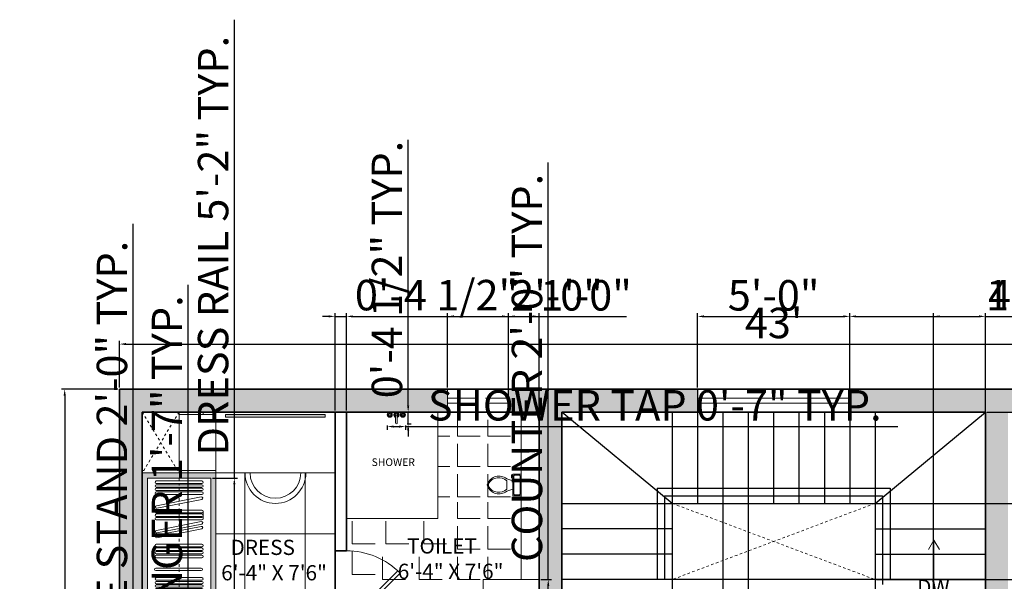
# Model space of a CAD drawing. Units: millimetres. Extents: x 542930 to 543750, y 628093 to 628738.
# Tile 7 of 14: x 542944 to 543333, y 628514 to 628735. Entities that reach past the tile are written whole.
import ezdxf

# ---------------------------------------------------------------- set-up
doc = ezdxf.new("R2010")
doc.units = ezdxf.units.MM
doc.linetypes.add('ACAD_ISO02W100', pattern=[15, 12, -3])
doc.linetypes.add('JIS_02_1.0', pattern=[2, 1, -1])
for name, color, linetype, lineweight in [('A-ANNO-DIMS', 2, 'Continuous', 18), ('A-ANNO-SYMB', 4, 'Continuous', 18), ('A-FLOR-FIXT', 9, 'Continuous', 18), ('A-FLOR-STRS', 7, 'Continuous', 25), ('A-FLOR-STRS-HIDN', 7, 'JIS_02_1.0', 13), ('A-FURN', 8, 'Continuous', 18), ('A-FURN-MILL', 8, 'Continuous', 18), ('A-FURN-MILL-HIDN', 8, 'JIS_02_1.0', 13), ('A-FURN-PATT', 9, 'Continuous', 13), ('A-GLAZ-HIDN', 70, 'ACAD_ISO02W100', 18), ('A-WALL', 7, 'Continuous', 35), ('DOORS', 30, 'Continuous', 18), ('WINDOW', 70, 'Continuous', 18)]:
    doc.layers.add(name, color=color, linetype=linetype, lineweight=lineweight)
for name, color, linetype, lineweight, true_color in [('A-ANNO-TEXT', 40, 'Continuous', 18, 0xf8d731), ('A-AREA-IDEN', 40, 'Continuous', 18, 0xf8d731), ('A-FLOR-PATT', 241, 'Continuous', 13, 0xf7abae), ('A-WALL-PATT', 251, 'Continuous', 13, 0x636466)]:
    doc.layers.add(name, color=color, linetype=linetype, lineweight=lineweight, true_color=true_color)
doc.styles.get("Standard").update_dxf_attribs({"font": 'arial.ttf'})
doc.dimstyles.new('ISO-25', dxfattribs={"dimtxt": 12, "dimasz": 2.5, "dimexe": 1.25, "dimexo": 0.625, "dimtad": 1, "dimdec": 0, "dimlunit": 3, "dimtxsty": 'Standard', "dimcen": 2.5, "dimadec": 0, "dimazin": 0, "dimtfac": 1, "dimtdec": 0, "dimtmove": 0, "dimatfit": 3, "dimfxl": 1, "dimarcsym": 0})

# ---------------------------------------------------------------- blocks, each defined once
blk = doc.blocks.new('*U3')
for p, q in [((-40, 0), (-40, -6)), ((0, 0), (0, -6))]:
    blk.add_line(p, q)
blk.add_lwpolyline([(0, 0), (-28.28, 28.28), (-29.52, 27.05), (-1.24, -1.24)], close=True)
blk.add_arc((0, 0), 40, 135, 180)
blk = doc.blocks.new('*U6')
for p, q in [((-10, -8.5), (-8, -8.5)), ((-10, -9.5), (-10, -8.5)), ((-7, -9.5), (-10, -9.5)), ((-8, -8.5), (-8, -8)), ((-7, -8), (-7, -9.5)), ((-4, -8), (-6, -14)), ((4, -8), (6, -14)), ((9.5, -6), (9.5, -2)), ((4, -14), (-4, -14))]:
    blk.add_line(p, q)
blk.add_lwpolyline([(10.5, -8), (10.5, 0), (-10.5, 0), (-10.5, -8)], close=True)
for points in [[(-9.5, -2), (-9.5, -6)], [(8.5, -1), (-8.5, -1)], [(-8.5, -7), (8.5, -7)]]:
    blk.add_lwpolyline(points)
for centre, radius, start, end in [((-8.62, -1.88), 0.884, 81.8699, 188.1301), ((-8.62, -6.12), 0.884, 171.8699, 278.1301), ((8.62, -1.88), 0.884, 351.8699, 98.1301), ((8.62, -6.12), 0.884, 261.8699, 8.1301), ((3.52, -21.58), 12.17, 141.46911, 247.97143), ((4.2, -21.82), 11.33, 136.36773, 238.94682), ((-3.52, -21.58), 12.17, 292.02843, 38.53071), ((-4.2, -21.82), 11.33, 301.05301, 43.63209), ((0, -27.88), 4, 245.73182, 294.26817), ((0, -29), 4, 254.86053, 285.13947)]:
    blk.add_arc(centre, radius, start, end)
blk = doc.blocks.new('Faucet - Bathroom top')
for p, q in [((-4.107, 0.125), (-4.375, 0.125)), ((-3.75, 0.4788), (-3.75, 0.75)), ((-3.5, 0.482), (-3.5, 0.75)), ((-3.1461, 0.125), (-2.875, 0.125)), ((3.143, 0.125), (2.875, 0.125)), ((3.5, 0.4788), (3.5, 0.75)), ((3.75, 0.482), (3.75, 0.75)), ((4.1039, 0.125), (4.375, 0.125)), ((-4.1039, -0.125), (-4.375, -0.125)), ((-3.75, -0.4821), (-3.75, -0.75)), ((-3.5, -0.4789), (-3.5, -0.75)), ((-3.143, -0.125), (-2.875, -0.125)), ((-0.5, -0.8639), (-0.5, -4.5)), ((0.5, -4.5), (0.5, -0.8631)), ((3.1461, -0.125), (2.875, -0.125)), ((3.5, -0.4821), (3.5, -0.75)), ((3.75, -0.4789), (3.75, -0.75)), ((4.107, -0.125), (4.375, -0.125))]:
    blk.add_line(p, q)
for centre, radius in [((-3.625, 0), 1.375), ((-4.625, 0), 0.2795), ((-3.625, 0), 0.5), ((-3.625, 1), 0.2795), ((-2.625, 0), 0.2795), ((0, 0), 0.5), ((3.625, 0), 1.375), ((2.625, 0), 0.2795), ((3.625, 0), 0.5), ((3.625, 1), 0.2795), ((4.625, 0), 0.2795), ((-3.625, -1), 0.2795), ((3.625, -1), 0.2795)]:
    blk.add_circle(centre, radius)
for centre, radius, start, end in [((-3.625, 0), 1, 105.2407, 164.2093), ((-3.625, 0), 1, 16.44125, 74.07887), ((0, 0), 1.5, 289.6514, 250.3603), ((0, 0), 1, 300.3431, 239.7554), ((3.625, 0), 1, 106.12, 164.0884), ((3.625, 0), 1, 16.23422, 73.90469), ((-3.625, 0), 1, 196.2342, 253.9047), ((-3.625, 0), 1, 286.12, 344.0884), ((0, -4.5), 0.5, 180, 0), ((3.625, 0), 1, 196.4413, 254.0789), ((3.625, 0), 1, 285.2407, 344.2093)]:
    blk.add_arc(centre, radius, start, end)
blk = doc.blocks.new('*D19')
at = {"layer": 'A-ANNO-DIMS', "color": 0, "lineweight": -2, "transparency": 16777216}
for p, q in [((542983.67, 628590.45), (542983.67, 628608.87)), ((542986.17, 628607.62), (543497.17, 628607.62)), ((543499.67, 628590.45), (543499.67, 628608.87))]:
    blk.add_line(p, q, dxfattribs=at)
at = {"layer": 'A-ANNO-DIMS', "color": 0, "transparency": 16777216}
for points in [[(542986.17, 628608.04), (542986.17, 628607.2), (542983.67, 628607.62)], [(543497.17, 628608.04), (543497.17, 628607.2), (543499.67, 628607.62)]]:
    blk.add_solid(points, dxfattribs=at)
at = {"layer": 'Defpoints', "color": 0, "transparency": 16777216}
for p in [(543499.67, 628607.62), (542983.67, 628589.83), (543499.67, 628589.83)]:
    blk.add_point(p, dxfattribs=at)
at = {"layer": 'A-ANNO-DIMS', "color": 0, "transparency": 16777216, "insert": (543241.67, 628614.38), "char_height": 12, "attachment_point": 5}
blk.add_mtext("43'", dxfattribs=at)
blk = doc.blocks.new('*D20')
at = {"layer": 'A-ANNO-DIMS', "color": 0, "lineweight": -2, "transparency": 16777216}
for p, q in [((542983.04, 628589.83), (542960.8, 628589.83)), ((542962.05, 628587.33), (542962.05, 628256.33)), ((542983.04, 628253.83), (542960.8, 628253.83))]:
    blk.add_line(p, q, dxfattribs=at)
at = {"layer": 'A-ANNO-DIMS', "color": 0, "transparency": 16777216}
for points in [[(542961.64, 628587.33), (542962.47, 628587.33), (542962.05, 628589.83)], [(542961.64, 628256.33), (542962.47, 628256.33), (542962.05, 628253.83)]]:
    blk.add_solid(points, dxfattribs=at)
at = {"layer": 'Defpoints', "color": 0, "transparency": 16777216}
for p in [(542983.67, 628589.83), (542962.05, 628253.83), (542983.67, 628253.83)]:
    blk.add_point(p, dxfattribs=at)
at = {"layer": 'A-ANNO-DIMS', "color": 0, "transparency": 16777216, "insert": (542955.3, 628421.83), "char_height": 12, "attachment_point": 5, "rotation": 90}
blk.add_mtext("28'", dxfattribs=at)
blk = doc.blocks.new('WARDROBE-DRESS-RAIL')
for p, q in [((0, 0), (0, 62)), ((0, 62), (25, 62)), ((3.52, 60.83), (21.52, 60.83)), ((3.52, 59.83), (21.52, 59.83)), ((3.52, 59.35), (21.52, 59.35)), ((3.52, 58.35), (21.52, 58.35)), ((25, 0), (25, 62)), ((3.52, 58.02), (21.52, 58.02)), ((3.52, 57.02), (21.52, 57.02)), ((3.52, 56.51), (21.52, 56.51)), ((3.52, 55.51), (21.52, 55.51)), ((3.57, 51.08), (21.23, 54.55)), ((3.76, 50.1), (21.43, 53.57)), ((3.52, 49.31), (21.52, 49.31)), ((3.52, 48.31), (21.52, 48.31)), ((3.52, 47.82), (21.52, 47.82)), ((3.52, 46.82), (21.52, 46.82)), ((3.52, 46.49), (21.52, 46.49)), ((3.52, 45.49), (21.52, 45.49)), ((3.57, 41.35), (21.23, 44.82)), ((3.57, 39.47), (21.23, 42.94)), ((3.76, 40.37), (21.43, 43.84)), ((3.76, 38.49), (21.43, 41.96)), ((3.52, 35.91), (21.52, 35.91)), ((3.52, 34.91), (21.52, 34.91)), ((3.52, 34.43), (21.52, 34.43)), ((3.52, 33.43), (21.52, 33.43)), ((3.52, 33.1), (21.52, 33.1)), ((3.52, 32.1), (21.52, 32.1)), ((3.52, 31.59), (21.52, 31.59)), ((3.52, 30.59), (21.52, 30.59)), ((3.27, 26.51), (21.27, 26.51)), ((3.27, 25.51), (21.27, 25.51)), ((3.52, 22.74), (21.52, 22.74)), ((3.52, 21.74), (21.52, 21.74)), ((3.52, 21.26), (21.52, 21.26)), ((3.52, 20.26), (21.52, 20.26)), ((3.52, 19.93), (21.52, 19.93)), ((3.52, 18.93), (21.52, 18.93)), ((3.52, 18.42), (21.52, 18.42)), ((3.52, 17.42), (21.52, 17.42)), ((3.56, 15.93), (21.44, 13.91)), ((3.27, 11.99), (21.27, 11.99)), ((3.44, 14.93), (21.33, 12.92)), ((3.27, 10.99), (21.27, 10.99)), ((3.52, 8.06), (21.52, 8.06)), ((3.52, 7.06), (21.52, 7.06)), ((3.52, 6.58), (21.52, 6.58)), ((3.52, 5.58), (21.52, 5.58)), ((3.52, 5.25), (21.52, 5.25)), ((3.52, 4.25), (21.52, 4.25)), ((3.52, 3.74), (21.52, 3.74)), ((3.52, 2.74), (21.52, 2.74)), ((0, 0), (25, 0))]:
    blk.add_line(p, q)
for centre, start, end in [((3.52, 60.33), 90, 270), ((3.52, 58.85), 90, 270), ((21.52, 60.33), 270, 90), ((21.52, 58.85), 270, 90), ((3.52, 57.52), 90, 270), ((3.52, 56.01), 90, 270), ((21.33, 54.06), 281.1082, 101.1082), ((21.52, 57.52), 270, 90), ((21.52, 56.01), 270, 90), ((3.67, 50.59), 101.1082, 281.1082), ((3.52, 48.81), 90, 270), ((3.52, 47.32), 90, 270), ((21.52, 48.81), 270, 90), ((21.52, 47.32), 270, 90), ((3.52, 45.99), 90, 270), ((21.33, 44.33), 281.1082, 101.1082), ((21.33, 42.45), 281.1082, 101.1082), ((21.52, 45.99), 270, 90), ((3.67, 40.86), 101.1082, 281.1082), ((3.67, 38.98), 101.1082, 281.1082), ((3.52, 35.41), 90, 270), ((21.52, 35.41), 270, 90), ((3.52, 33.93), 90, 270), ((3.52, 32.6), 90, 270), ((3.52, 31.09), 90, 270), ((21.52, 33.93), 270, 90), ((21.52, 32.6), 270, 90), ((21.52, 31.09), 270, 90), ((3.27, 26.01), 90, 270), ((21.27, 26.01), 270, 90), ((3.52, 22.24), 90, 270), ((3.52, 20.76), 90, 270), ((3.52, 19.43), 90, 270), ((21.52, 22.24), 270, 90), ((21.52, 20.76), 270, 90), ((21.52, 19.43), 270, 90), ((3.5, 15.43), 83.5593, 263.5593), ((3.52, 17.92), 90, 270), ((21.52, 17.92), 270, 90), ((3.27, 11.49), 90, 270), ((21.27, 11.49), 270, 90), ((21.39, 13.41), 263.5593, 83.5611), ((3.52, 7.56), 90, 270), ((21.52, 7.56), 270, 90), ((3.52, 6.08), 90, 270), ((3.52, 4.75), 90, 270), ((21.52, 6.08), 270, 90), ((21.52, 4.75), 270, 90), ((3.52, 3.24), 90, 270), ((21.52, 3.24), 270, 90)]:
    blk.add_arc(centre, 0.5, start, end)
blk = doc.blocks.new('SHOWER-ENCLOSURE')
for p, q in [((36, 0), (36, 42)), ((0, 0), (36, 0))]:
    blk.add_line(p, q)
blk = doc.blocks.new('LAVATORY-COUNTER')
for p, q in [((0, 0), (0, 24)), ((0, 24), (22, 24))]:
    blk.add_line(p, q)
blk = doc.blocks.new('DRESSING-STOOL')
for radius in [12, 10]:
    blk.add_arc((12, 12), radius, 180, 0)
blk = doc.blocks.new('*D31')
at = {"layer": 'A-ANNO-DIMS', "color": 0, "lineweight": -2, "transparency": 16777216}
for p, q in [((543010.77, 628478.3), (543010.77, 628630.92)), ((543012.99, 628478.3), (543009.52, 628478.3)), ((543010.77, 628461.8), (543010.77, 628475.8)), ((543012.99, 628459.3), (543009.52, 628459.3))]:
    blk.add_line(p, q, dxfattribs=at)
at = {"layer": 'A-ANNO-DIMS', "color": 0, "transparency": 16777216}
for points in [[(543010.35, 628475.8), (543011.18, 628475.8), (543010.77, 628478.3)], [(543010.35, 628461.8), (543011.18, 628461.8), (543010.77, 628459.3)]]:
    blk.add_solid(points, dxfattribs=at)
at = {"layer": 'Defpoints', "color": 0, "transparency": 16777216}
for p in [(543010.77, 628478.3), (543013.62, 628478.3), (543013.62, 628459.3)]:
    blk.add_point(p, dxfattribs=at)
at = {"layer": 'A-ANNO-DIMS', "color": 0, "transparency": 16777216, "insert": (543003.94, 628555.86), "char_height": 12, "attachment_point": 5, "rotation": 90}
blk.add_mtext('HANGER 1\'-7" TYP.', dxfattribs=at)
blk = doc.blocks.new('*D39')
at = {"layer": 'A-ANNO-DIMS', "color": 0, "lineweight": -2, "transparency": 16777216}
for p, q in [((543089.3, 628575.56), (543089.3, 628573.86)), ((543091.8, 628575.11), (543093.95, 628575.11)), ((543096.45, 628575.56), (543096.45, 628573.86)), ((543096.45, 628575.11), (543290.64, 628575.11))]:
    blk.add_line(p, q, dxfattribs=at)
at = {"layer": 'A-ANNO-DIMS', "color": 0, "transparency": 16777216}
for points in [[(543091.8, 628575.52), (543091.8, 628574.69), (543089.3, 628575.11)], [(543093.95, 628575.52), (543093.95, 628574.69), (543096.45, 628575.11)]]:
    blk.add_solid(points, dxfattribs=at)
at = {"layer": 'Defpoints', "color": 0, "transparency": 16777216}
for p in [(543089.3, 628576.18), (543096.45, 628576.18), (543096.45, 628575.11)]:
    blk.add_point(p, dxfattribs=at)
at = {"layer": 'A-ANNO-DIMS', "color": 0, "transparency": 16777216, "insert": (543194.79, 628581.94), "char_height": 12, "attachment_point": 5}
blk.add_mtext('SHOWER TAP 0\'-7" TYP.', dxfattribs=at)
blk = doc.blocks.new('*D40')
at = {"layer": 'A-ANNO-DIMS', "color": 0, "lineweight": -2, "transparency": 16777216}
for p, q in [((543097.52, 628583.33), (543097.52, 628688.18)), ((543097.07, 628580.83), (543098.77, 628580.83)), ((543097.52, 628576.18), (543097.52, 628580.83)), ((543097.07, 628576.18), (543098.77, 628576.18)), ((543097.52, 628573.68), (543097.52, 628571.18))]:
    blk.add_line(p, q, dxfattribs=at)
at = {"layer": 'A-ANNO-DIMS', "color": 0, "transparency": 16777216}
for points in [[(543097.1, 628583.33), (543097.94, 628583.33), (543097.52, 628580.83)], [(543097.1, 628573.68), (543097.94, 628573.68), (543097.52, 628576.18)]]:
    blk.add_solid(points, dxfattribs=at)
at = {"layer": 'Defpoints', "color": 0, "transparency": 16777216}
for p in [(543096.45, 628580.83), (543097.52, 628580.83), (543096.45, 628576.18)]:
    blk.add_point(p, dxfattribs=at)
at = {"layer": 'A-ANNO-DIMS', "color": 0, "transparency": 16777216, "insert": (543090.69, 628637), "char_height": 12, "attachment_point": 5, "rotation": 90}
blk.add_mtext('0\'-4 1/2" TYP.', dxfattribs=at)
blk = doc.blocks.new('*D43')
at = {"layer": 'A-ANNO-DIMS', "color": 0, "lineweight": -2, "transparency": 16777216}
for p, q in [((543028.97, 628554.83), (543028.97, 628735.47)), ((543020.29, 628554.83), (543030.22, 628554.83)), ((543028.97, 628495.33), (543028.97, 628552.33)), ((543020.29, 628492.83), (543030.22, 628492.83))]:
    blk.add_line(p, q, dxfattribs=at)
at = {"layer": 'A-ANNO-DIMS', "color": 0, "transparency": 16777216}
for points in [[(543028.55, 628552.33), (543029.38, 628552.33), (543028.97, 628554.83)], [(543028.55, 628495.33), (543029.38, 628495.33), (543028.97, 628492.83)]]:
    blk.add_solid(points, dxfattribs=at)
at = {"layer": 'Defpoints', "color": 0, "transparency": 16777216}
for p in [(543019.67, 628554.83), (543028.97, 628554.83), (543019.67, 628492.83)]:
    blk.add_point(p, dxfattribs=at)
at = {"layer": 'A-ANNO-DIMS', "color": 0, "transparency": 16777216, "insert": (543022.14, 628646.4), "char_height": 12, "attachment_point": 5, "rotation": 90}
blk.add_mtext('DRESS RAIL 5\'-2" TYP.', dxfattribs=at)
blk = doc.blocks.new('*D55')
at = {"layer": 'A-ANNO-DIMS', "color": 0, "lineweight": -2, "transparency": 16777216}
for p, q in [((543152.77, 628514.83), (543152.77, 628679.13)), ((543149.79, 628514.83), (543154.02, 628514.83)), ((543152.77, 628493.33), (543152.77, 628512.33)), ((543149.79, 628490.83), (543154.02, 628490.83))]:
    blk.add_line(p, q, dxfattribs=at)
at = {"layer": 'A-ANNO-DIMS', "color": 0, "transparency": 16777216}
for points in [[(543152.35, 628512.33), (543153.18, 628512.33), (543152.77, 628514.83)], [(543152.35, 628493.33), (543153.18, 628493.33), (543152.77, 628490.83)]]:
    blk.add_solid(points, dxfattribs=at)
at = {"layer": 'Defpoints', "color": 0, "transparency": 16777216}
for p in [(543149.17, 628514.83), (543152.77, 628514.83), (543149.17, 628490.83)]:
    blk.add_point(p, dxfattribs=at)
at = {"layer": 'A-ANNO-DIMS', "color": 0, "transparency": 16777216, "insert": (543145.93, 628598.23), "char_height": 12, "attachment_point": 5, "rotation": 90}
blk.add_mtext('COUNTER 2\'-0" TYP.', dxfattribs=at)
blk = doc.blocks.new('*D59')
at = {"layer": 'A-ANNO-DIMS', "color": 0, "lineweight": -2, "transparency": 16777216}
for p, q in [((542989.07, 628438.89), (542989.07, 628654.99)), ((542992.04, 628438.89), (542987.82, 628438.89)), ((542989.07, 628417.39), (542989.07, 628436.39)), ((542992.04, 628414.89), (542987.82, 628414.89))]:
    blk.add_line(p, q, dxfattribs=at)
at = {"layer": 'A-ANNO-DIMS', "color": 0, "transparency": 16777216}
for points in [[(542988.65, 628436.39), (542989.48, 628436.39), (542989.07, 628438.89)], [(542988.65, 628417.39), (542989.48, 628417.39), (542989.07, 628414.89)]]:
    blk.add_solid(points, dxfattribs=at)
at = {"layer": 'Defpoints', "color": 0, "transparency": 16777216}
for p in [(542989.07, 628438.89), (542992.67, 628438.89), (542992.67, 628414.89)]:
    blk.add_point(p, dxfattribs=at)
at = {"layer": 'A-ANNO-DIMS', "color": 0, "transparency": 16777216, "insert": (542982.24, 628548.19), "char_height": 12, "attachment_point": 5, "rotation": 90}
blk.add_mtext('BEDSIDE STAND 2\'-0" TYP.', dxfattribs=at)
blk = doc.blocks.new('*D66')
at = {"layer": 'A-ANNO-DIMS', "color": 0, "lineweight": -2, "transparency": 16777216}
for p, q in [((543113.07, 628590.45), (543113.07, 628619.78)), ((543137.07, 628590.45), (543137.07, 628619.78)), ((543115.57, 628618.53), (543134.57, 628618.53)), ((543137.07, 628618.53), (543172.92, 628618.53))]:
    blk.add_line(p, q, dxfattribs=at)
at = {"layer": 'A-ANNO-DIMS', "color": 0, "transparency": 16777216}
for points in [[(543115.57, 628618.94), (543115.57, 628618.11), (543113.07, 628618.53)], [(543134.57, 628618.94), (543134.57, 628618.11), (543137.07, 628618.53)]]:
    blk.add_solid(points, dxfattribs=at)
at = {"layer": 'Defpoints', "color": 0, "transparency": 16777216}
for p in [(543137.07, 628618.53), (543113.07, 628589.83), (543137.07, 628589.83)]:
    blk.add_point(p, dxfattribs=at)
at = {"layer": 'A-ANNO-DIMS', "color": 0, "transparency": 16777216, "insert": (543156.24, 628625.28), "char_height": 12, "attachment_point": 5}
blk.add_mtext('2\'-0"', dxfattribs=at)
blk = doc.blocks.new('*D67')
at = {"layer": 'A-ANNO-DIMS', "color": 0, "lineweight": -2, "transparency": 16777216}
for p, q in [((543137.07, 628581.45), (543137.07, 628619.78)), ((543149.17, 628581.45), (543149.17, 628619.78)), ((543139.57, 628618.53), (543146.67, 628618.53)), ((543149.17, 628618.53), (543183.69, 628618.53))]:
    blk.add_line(p, q, dxfattribs=at)
at = {"layer": 'A-ANNO-DIMS', "color": 0, "transparency": 16777216}
for points in [[(543139.57, 628618.94), (543139.57, 628618.11), (543137.07, 628618.53)], [(543146.67, 628618.94), (543146.67, 628618.11), (543149.17, 628618.53)]]:
    blk.add_solid(points, dxfattribs=at)
at = {"layer": 'Defpoints', "color": 0, "transparency": 16777216}
for p in [(543149.17, 628618.53), (543137.07, 628580.83), (543149.17, 628580.83)]:
    blk.add_point(p, dxfattribs=at)
at = {"layer": 'A-ANNO-DIMS', "color": 0, "transparency": 16777216, "insert": (543167.68, 628625.28), "char_height": 12, "attachment_point": 5}
blk.add_mtext('1\'-0"', dxfattribs=at)
blk = doc.blocks.new('*D68')
at = {"layer": 'A-ANNO-DIMS', "color": 0, "lineweight": -2, "transparency": 16777216}
for p, q in [((543211.67, 628590.45), (543211.67, 628619.78)), ((543271.67, 628590.45), (543271.67, 628619.78)), ((543214.17, 628618.53), (543269.17, 628618.53))]:
    blk.add_line(p, q, dxfattribs=at)
at = {"layer": 'A-ANNO-DIMS', "color": 0, "transparency": 16777216}
for points in [[(543214.17, 628618.94), (543214.17, 628618.11), (543211.67, 628618.53)], [(543269.17, 628618.94), (543269.17, 628618.11), (543271.67, 628618.53)]]:
    blk.add_solid(points, dxfattribs=at)
at = {"layer": 'Defpoints', "color": 0, "transparency": 16777216}
for p in [(543271.67, 628618.53), (543211.67, 628589.83), (543271.67, 628589.83)]:
    blk.add_point(p, dxfattribs=at)
at = {"layer": 'A-ANNO-DIMS', "color": 0, "transparency": 16777216, "insert": (543241.67, 628625.28), "char_height": 12, "attachment_point": 5}
blk.add_mtext('5\'-0"', dxfattribs=at)
blk = doc.blocks.new('*D69')
at = {"layer": 'A-ANNO-DIMS', "color": 0, "lineweight": -2, "transparency": 16777216}
for p, q in [((543271.67, 628584.95), (543271.67, 628619.78)), ((543325.17, 628581.45), (543325.17, 628619.78)), ((543274.17, 628618.53), (543322.67, 628618.53)), ((543325.17, 628618.53), (543389.26, 628618.53))]:
    blk.add_line(p, q, dxfattribs=at)
at = {"layer": 'A-ANNO-DIMS', "color": 0, "transparency": 16777216}
for points in [[(543274.17, 628618.94), (543274.17, 628618.11), (543271.67, 628618.53)], [(543322.67, 628618.94), (543322.67, 628618.11), (543325.17, 628618.53)]]:
    blk.add_solid(points, dxfattribs=at)
at = {"layer": 'Defpoints', "color": 0, "transparency": 16777216}
for p in [(543325.17, 628618.53), (543271.67, 628584.33), (543325.17, 628580.83)]:
    blk.add_point(p, dxfattribs=at)
at = {"layer": 'A-ANNO-DIMS', "color": 0, "transparency": 16777216, "insert": (543358.46, 628625.36), "char_height": 12, "attachment_point": 5}
blk.add_mtext('4\'-5 1/2"', dxfattribs=at)
blk = doc.blocks.new('*D70')
at = {"layer": 'A-ANNO-DIMS', "color": 0, "lineweight": -2, "transparency": 16777216}
for p, q in [((543325.79, 628580.83), (543537.81, 628580.83)), ((543536.56, 628517.33), (543536.56, 628578.33)), ((543325.79, 628514.83), (543537.81, 628514.83))]:
    blk.add_line(p, q, dxfattribs=at)
at = {"layer": 'A-ANNO-DIMS', "color": 0, "transparency": 16777216}
for points in [[(543536.15, 628578.33), (543536.98, 628578.33), (543536.56, 628580.83)], [(543536.15, 628517.33), (543536.98, 628517.33), (543536.56, 628514.83)]]:
    blk.add_solid(points, dxfattribs=at)
at = {"layer": 'Defpoints', "color": 0, "transparency": 16777216}
for p in [(543325.17, 628580.83), (543536.56, 628580.83), (543325.17, 628514.83)]:
    blk.add_point(p, dxfattribs=at)
at = {"layer": 'A-ANNO-DIMS', "color": 0, "transparency": 16777216, "insert": (543529.81, 628547.83), "char_height": 12, "attachment_point": 5, "rotation": 90}
blk.add_mtext('5\'-6"', dxfattribs=at)
blk = doc.blocks.new('*D71')
at = {"layer": 'A-ANNO-DIMS', "color": 0, "lineweight": -2, "transparency": 16777216}
for p, q in [((543201.67, 628544.2), (543201.67, 628103.84)), ((543281.67, 628544.2), (543281.67, 628103.84)), ((543204.17, 628105.09), (543279.17, 628105.09))]:
    blk.add_line(p, q, dxfattribs=at)
at = {"layer": 'A-ANNO-DIMS', "color": 0, "transparency": 16777216}
for points in [[(543204.17, 628105.5), (543204.17, 628104.67), (543201.67, 628105.09)], [(543279.17, 628105.5), (543279.17, 628104.67), (543281.67, 628105.09)]]:
    blk.add_solid(points, dxfattribs=at)
at = {"layer": 'Defpoints', "color": 0, "transparency": 16777216}
for p in [(543201.67, 628544.83), (543281.67, 628544.83), (543281.67, 628105.09)]:
    blk.add_point(p, dxfattribs=at)
at = {"layer": 'A-ANNO-DIMS', "color": 0, "transparency": 16777216, "insert": (543241.67, 628111.84), "char_height": 12, "attachment_point": 5}
blk.add_mtext('6\'-8"', dxfattribs=at)
blk = doc.blocks.new('*D72')
at = {"layer": 'A-ANNO-DIMS', "color": 0, "lineweight": -2, "transparency": 16777216}
for p, q in [((543536.56, 628544.83), (543536.56, 628580.68)), ((543282.29, 628544.83), (543537.81, 628544.83)), ((543536.56, 628517.33), (543536.56, 628542.33)), ((543282.29, 628514.83), (543537.81, 628514.83))]:
    blk.add_line(p, q, dxfattribs=at)
at = {"layer": 'A-ANNO-DIMS', "color": 0, "transparency": 16777216}
for points in [[(543536.15, 628542.33), (543536.98, 628542.33), (543536.56, 628544.83)], [(543536.15, 628517.33), (543536.98, 628517.33), (543536.56, 628514.83)]]:
    blk.add_solid(points, dxfattribs=at)
at = {"layer": 'Defpoints', "color": 0, "transparency": 16777216}
for p in [(543281.67, 628544.83), (543536.56, 628544.83), (543281.67, 628514.83)]:
    blk.add_point(p, dxfattribs=at)
at = {"layer": 'A-ANNO-DIMS', "color": 0, "transparency": 16777216, "insert": (543529.81, 628564), "char_height": 12, "attachment_point": 5, "rotation": 90}
blk.add_mtext('2\'-6"', dxfattribs=at)
blk = doc.blocks.new('*D78')
at = {"layer": 'A-ANNO-DIMS', "color": 0, "lineweight": -2, "transparency": 16777216}
for p, q in [((543304.67, 628350.45), (543304.67, 628619.78)), ((543325.17, 628350.45), (543325.17, 628619.78)), ((543307.17, 628618.53), (543322.67, 628618.53)), ((543325.17, 628618.53), (543387.65, 628618.53))]:
    blk.add_line(p, q, dxfattribs=at)
at = {"layer": 'A-ANNO-DIMS', "color": 0, "transparency": 16777216}
for points in [[(543307.17, 628618.94), (543307.17, 628618.11), (543304.67, 628618.53)], [(543322.67, 628618.94), (543322.67, 628618.11), (543325.17, 628618.53)]]:
    blk.add_solid(points, dxfattribs=at)
at = {"layer": 'Defpoints', "color": 0, "transparency": 16777216}
for p in [(543325.17, 628618.53), (543304.67, 628349.83), (543325.17, 628349.83)]:
    blk.add_point(p, dxfattribs=at)
at = {"layer": 'A-ANNO-DIMS', "color": 0, "transparency": 16777216, "insert": (543357.66, 628625.36), "char_height": 12, "attachment_point": 5}
blk.add_mtext('1\'-8 1/2"', dxfattribs=at)
blk = doc.blocks.new('*D86')
at = {"layer": 'A-ANNO-DIMS', "color": 0, "lineweight": -2, "transparency": 16777216}
for p, q in [((543068.67, 628581.45), (543068.67, 628619.78)), ((543073.17, 628581.45), (543073.17, 628619.78)), ((543066.17, 628618.53), (543063.67, 628618.53)), ((543068.67, 628618.53), (543073.17, 628618.53)), ((543075.67, 628618.53), (543139.28, 628618.53))]:
    blk.add_line(p, q, dxfattribs=at)
at = {"layer": 'A-ANNO-DIMS', "color": 0, "transparency": 16777216}
for points in [[(543066.17, 628618.94), (543066.17, 628618.11), (543068.67, 628618.53)], [(543075.67, 628618.94), (543075.67, 628618.11), (543073.17, 628618.53)]]:
    blk.add_solid(points, dxfattribs=at)
at = {"layer": 'Defpoints', "color": 0, "transparency": 16777216}
for p in [(543073.17, 628618.53), (543068.67, 628580.83), (543073.17, 628580.83)]:
    blk.add_point(p, dxfattribs=at)
at = {"layer": 'A-ANNO-DIMS', "color": 0, "transparency": 16777216, "insert": (543108.72, 628625.36), "char_height": 12, "attachment_point": 5}
blk.add_mtext('0\'-4 1/2"', dxfattribs=at)
blk = doc.blocks.new('*D87')
at = {"layer": 'A-ANNO-DIMS', "color": 0, "lineweight": -2, "transparency": 16777216}
for p, q in [((543221.67, 628580.2), (543221.67, 628103.84)), ((543231.67, 628580.2), (543231.67, 628103.84)), ((543224.17, 628105.09), (543229.17, 628105.09)), ((543231.67, 628105.09), (543276.64, 628105.09))]:
    blk.add_line(p, q, dxfattribs=at)
at = {"layer": 'A-ANNO-DIMS', "color": 0, "transparency": 16777216}
for points in [[(543224.17, 628105.5), (543224.17, 628104.67), (543221.67, 628105.09)], [(543229.17, 628105.5), (543229.17, 628104.67), (543231.67, 628105.09)]]:
    blk.add_solid(points, dxfattribs=at)
at = {"layer": 'Defpoints', "color": 0, "transparency": 16777216}
for p in [(543221.67, 628580.83), (543231.67, 628580.83), (543231.67, 628105.09)]:
    blk.add_point(p, dxfattribs=at)
at = {"layer": 'A-ANNO-DIMS', "color": 0, "transparency": 16777216, "insert": (543255.4, 628111.84), "char_height": 12, "attachment_point": 5}
blk.add_mtext('0\'-10"', dxfattribs=at)

msp = doc.modelspace()

# ---------------------------------------------------------------- hatches: boundary and pattern name
at = {"layer": 'A-FURN-PATT'}
h = msp.add_hatch(color=256, dxfattribs=at)
h.dxf.hatch_style = 1
h.paths.add_polyline_path([(543064.84, 628579.83), (543025.49, 628579.83), (543025.49, 628578.83), (543064.84, 628578.83)])
h = msp.add_hatch(color=256, dxfattribs=at)
h.dxf.hatch_style = 1
h.paths.add_polyline_path([(543021.67, 628556.83), (542992.67, 628556.83), (542992.67, 628490.83), (543021.67, 628490.83)])
h.paths.add_polyline_path([(543019.67, 628492.83), (542994.67, 628492.83), (542994.67, 628554.83), (543019.67, 628554.83)], flags=16)
h.paths.add_polyline_path([(543016.19, 628514.57), (543007.17, 628514.57), (543007.17, 628514.08), (543016.19, 628514.08, -1), (543016.19, 628513.08), (543007.17, 628513.08), (543007.17, 628512.76), (543016.19, 628512.76, -1), (543016.19, 628511.76), (543007.17, 628511.76), (543007.17, 628511.24), (543016.19, 628511.24, -1), (543016.19, 628510.24), (543007.17, 628510.24), (543007.17, 628507.74), (543016.11, 628506.73, -1.000001), (543016, 628505.74), (543007.17, 628506.74), (543007.17, 628504.81), (543015.94, 628504.81, -1), (543015.94, 628503.81), (543007.17, 628503.81), (543007.17, 628500.89), (543016.19, 628500.89, -1), (543016.19, 628499.89), (543007.17, 628499.89), (543007.17, 628499.4), (543016.19, 628499.4, -1), (543016.19, 628498.4), (543007.17, 628498.4), (543007.17, 628498.08), (543016.19, 628498.08, -1), (543016.19, 628497.08), (543007.17, 628497.08), (543007.17, 628496.56), (543016.19, 628496.56, -1), (543016.19, 628495.56), (542998.19, 628495.56, -1), (542998.19, 628496.56), (543007.17, 628496.56), (543007.17, 628497.08), (542998.19, 628497.08, -1), (542998.19, 628498.08), (543007.17, 628498.08), (543007.17, 628498.4), (542998.19, 628498.4, -1), (542998.19, 628499.4), (543007.17, 628499.4), (543007.17, 628499.89), (542998.19, 628499.89, -1), (542998.19, 628500.89), (543007.17, 628500.89), (543007.17, 628503.81), (542997.94, 628503.81, -1), (542997.94, 628504.81), (543007.17, 628504.81), (543007.17, 628506.74), (542998.11, 628507.76, -0.999984), (542998.22, 628508.75), (543007.17, 628507.74), (543007.17, 628510.24), (542998.19, 628510.24, -1), (542998.19, 628511.24), (543007.17, 628511.24), (543007.17, 628511.76), (542998.19, 628511.76, -1), (542998.19, 628512.76), (543007.17, 628512.76), (543007.17, 628513.08), (542998.19, 628513.08, -1), (542998.19, 628514.08), (543007.17, 628514.08), (543007.17, 628514.57), (542998.19, 628514.57, -1), (542998.19, 628515.57), (543007.17, 628515.57), (543007.17, 628518.34), (542997.94, 628518.34, -1), (542997.94, 628519.34), (543007.17, 628519.34), (543007.17, 628523.41), (542998.19, 628523.41, -1), (542998.19, 628524.41), (543007.17, 628524.41), (543007.17, 628524.93), (542998.19, 628524.93, -1), (542998.19, 628525.93), (543007.17, 628525.93), (543007.17, 628526.25), (542998.19, 628526.25, -1), (542998.19, 628527.25), (543007.17, 628527.25), (543007.17, 628527.74), (542998.19, 628527.74, -1), (542998.19, 628528.74), (543007.17, 628528.74), (543007.17, 628533.03), (542998.43, 628531.31, -1.000015), (542998.24, 628532.29), (543007.17, 628534.05), (543007.17, 628534.91), (542998.43, 628533.2, -1.000015), (542998.24, 628534.18), (543007.17, 628535.93), (543007.17, 628538.32), (542998.19, 628538.32, -1), (542998.19, 628539.32), (543007.17, 628539.32), (543007.17, 628539.65), (542998.19, 628539.65, -1), (542998.19, 628540.65), (543007.17, 628540.65), (543007.17, 628541.13), (542998.19, 628541.13, -1), (542998.19, 628542.13), (543007.17, 628542.13), (543007.17, 628544.64), (542998.43, 628542.93, -1.000015), (542998.24, 628543.91), (543007.17, 628545.66), (543007.17, 628548.33), (542998.19, 628548.33, -1), (542998.19, 628549.33), (543007.17, 628549.33), (543007.17, 628549.84), (542998.19, 628549.84, -1), (542998.19, 628550.84), (543007.17, 628550.84), (543007.17, 628551.17), (542998.19, 628551.17, -1), (542998.19, 628552.17), (543007.17, 628552.17), (543007.17, 628552.66), (542998.19, 628552.66, -1), (542998.19, 628553.66), (543016.19, 628553.66, -1), (543016.19, 628552.66), (543007.17, 628552.66), (543007.17, 628552.17), (543016.19, 628552.17, -1), (543016.19, 628551.17), (543007.17, 628551.17), (543007.17, 628550.84), (543016.19, 628550.84, -1), (543016.19, 628549.84), (543007.17, 628549.84), (543007.17, 628549.33), (543016.19, 628549.33, -1), (543016.19, 628548.33), (543007.17, 628548.33), (543007.17, 628545.66), (543015.9, 628547.38, -1.000014), (543016.09, 628546.4), (543007.17, 628544.64), (543007.17, 628542.13), (543016.19, 628542.13, -0.50839), (543016.67, 628541.48), (543016.67, 628540.3, -0.156536), (543016.67, 628539.99), (543016.67, 628538.97, -0.50839), (543016.19, 628538.32), (543007.17, 628538.32), (543007.17, 628535.93), (543015.9, 628537.65, -1.000014), (543016.09, 628536.67), (543007.17, 628534.91), (543007.17, 628534.05), (543015.9, 628535.76, -1.000014), (543016.09, 628534.78), (543007.17, 628533.03), (543007.17, 628528.74), (543016.19, 628528.74, -1), (543016.19, 628527.74), (543007.17, 628527.74), (543007.17, 628527.25), (543016.19, 628527.25, -1), (543016.19, 628526.25), (543007.17, 628526.25), (543007.17, 628525.93), (543016.19, 628525.93, -1), (543016.19, 628524.93), (543007.17, 628524.93), (543007.17, 628524.41), (543016.19, 628524.41, -1), (543016.19, 628523.41), (543007.17, 628523.41), (543007.17, 628519.34), (543015.94, 628519.34, -1), (543015.94, 628518.34), (543007.17, 628518.34), (543007.17, 628515.57), (543016.19, 628515.57, -1)], flags=0)
at = {"layer": 'A-WALL-PATT'}
h = msp.add_hatch(color=256, dxfattribs=at)
h.dxf.hatch_style = 1
h.paths.add_polyline_path([(542992.67, 628481.83), (543028.62, 628481.83), (543028.62, 628490.83), (542992.67, 628490.83), (542992.67, 628580.83), (543113.07, 628580.83), (543113.07, 628589.83), (542983.67, 628589.83), (542983.67, 628335.3), (542992.67, 628335.3)])
h = msp.add_hatch(color=256, dxfattribs=at)
h.dxf.hatch_style = 1
h.paths.add_polyline_path([(543158.17, 628580.83), (543211.67, 628580.83), (543211.67, 628589.83), (543137.07, 628589.83), (543137.07, 628580.83), (543149.17, 628580.83), (543149.17, 628490.83), (543073.17, 628490.83), (543073.17, 628496.14), (543068.67, 628496.14), (543068.67, 628490.83), (543064.67, 628490.83), (543064.67, 628481.83), (543149.17, 628481.83), (543149.17, 628396.23), (543158.17, 628396.23)])
h = msp.add_hatch(color=256, dxfattribs=at)
h.dxf.hatch_style = 1
h.paths.add_polyline_path([(543454.53, 628589.83), (543271.67, 628589.83), (543271.67, 628580.83), (543325.17, 628580.83), (543325.17, 628475.36), (543334.17, 628475.36), (543334.17, 628481.83), (543370.17, 628481.83), (543370.17, 628490.83), (543334.17, 628490.83), (543334.17, 628580.83), (543410.17, 628580.83), (543410.17, 628524.86), (543414.67, 628524.86), (543414.67, 628580.83), (543454.53, 628580.83)])

# ---------------------------------------------------------------- linework, layer by layer
at = {"layer": 'A-ANNO-SYMB'}
for p, q in [((543304.92, 628530.28), (543302.71, 628526.7)), ((543304.92, 628514.83), (543304.92, 628530.28)), ((543304.92, 628530.28), (543307.13, 628526.7))]:
    msp.add_line(p, q, dxfattribs=at)
at = {"layer": 'A-FLOR-FIXT'}
msp.add_line((543142.07, 628514.83), (543142.07, 628580.83), dxfattribs=at)
at = {"layer": 'A-FLOR-PATT'}
for p, q in [((543016.67, 628579.83), (543016.67, 628580.83)), ((543116.93, 628577.8), (543116.93, 628571.36)), ((543128.93, 628577.8), (543128.93, 628571.36)), ((543109.17, 628571.36), (543113.93, 628571.36)), ((543116.93, 628571.36), (543125.93, 628571.36)), ((543116.93, 628568.36), (543116.93, 628559.36)), ((543128.93, 628571.36), (543137.93, 628571.36)), ((543128.93, 628568.36), (543128.93, 628559.36)), ((543033.13, 628424.06), (543033.13, 628556.83)), ((543056.96, 628424.17), (543056.96, 628556.83)), ((543109.17, 628559.36), (543113.93, 628559.36)), ((543116.93, 628559.36), (543125.93, 628559.36)), ((543128.93, 628559.36), (543137.93, 628559.36)), ((543116.93, 628556.36), (543116.93, 628547.36)), ((543128.93, 628556.36), (543128.93, 628547.36)), ((543109.17, 628547.36), (543113.93, 628547.36)), ((543116.93, 628547.36), (543125.93, 628547.36)), ((543116.93, 628545.27), (543116.93, 628538.83)), ((543128.93, 628547.36), (543137.93, 628547.36)), ((543128.93, 628545.27), (543128.93, 628538.83)), ((543016.67, 628538.67), (543016.67, 628541.79)), ((543075.49, 628537.86), (543075.49, 628528.86)), ((543088.75, 628537.86), (543088.75, 628528.86)), ((543103.68, 628537.86), (543103.68, 628528.86)), ((543116.93, 628538.83), (543125.93, 628538.83)), ((543128.93, 628538.83), (543137.93, 628538.83)), ((543116.93, 628535.83), (543116.93, 628526.83)), ((543128.93, 628535.83), (543128.93, 628526.83)), ((543021.67, 628532.83), (543068.67, 628532.83)), ((543075.49, 628528.86), (543084.49, 628528.86)), ((543075.49, 628525.86), (543075.49, 628516.86)), ((543088.75, 628528.86), (543097.75, 628528.86)), ((543103.68, 628528.86), (543112.68, 628528.86)), ((543116.93, 628526.83), (543125.93, 628526.83)), ((543128.93, 628526.83), (543137.93, 628526.83)), ((543087.43, 628523.83), (543087.43, 628514.83)), ((543101.92, 628523.83), (543101.92, 628514.83)), ((543116.93, 628523.83), (543116.93, 628514.83)), ((543128.93, 628523.83), (543128.93, 628514.83)), ((543116.93, 628521.27), (543116.93, 628514.83)), ((543075.49, 628516.86), (543084.49, 628516.86)), ((543087.43, 628514.83), (543096.43, 628514.83)), ((543101.92, 628514.83), (543110.92, 628514.83)), ((543116.93, 628514.83), (543125.93, 628514.83))]:
    msp.add_line(p, q, dxfattribs=at)
at = {"layer": 'A-FLOR-STRS'}
for p, q in [((543211.67, 628589.83), (543211.67, 628544.83)), ((543271.67, 628589.83), (543271.67, 628544.83)), ((543201.67, 628544.83), (543158.17, 628580.83)), ((543201.67, 628580.83), (543201.67, 628544.83)), ((543221.67, 628580.83), (543221.67, 628544.83)), ((543231.67, 628580.83), (543231.67, 628544.83)), ((543241.67, 628580.83), (543241.67, 628544.83)), ((543251.67, 628580.83), (543251.67, 628544.83)), ((543261.67, 628580.83), (543261.67, 628544.83)), ((543281.67, 628580.83), (543281.67, 628544.83)), ((543281.67, 628544.83), (543325.17, 628580.83)), ((543195.67, 628550.83), (543287.67, 628550.83)), ((543195.67, 628550.83), (543195.67, 628514.83)), ((543287.67, 628550.83), (543287.67, 628514.83)), ((543198.67, 628547.83), (543198.67, 628514.83)), ((543198.67, 628547.83), (543284.67, 628547.83)), ((543284.67, 628547.83), (543284.67, 628512.83)), ((543158.17, 628544.83), (543325.17, 628544.83)), ((543201.67, 628544.83), (543201.67, 628514.83)), ((543281.67, 628544.83), (543281.67, 628514.83)), ((543201.67, 628534.83), (543158.17, 628534.83)), ((543281.67, 628534.83), (543325.17, 628534.83)), ((543201.67, 628524.83), (543158.17, 628524.83)), ((543281.67, 628524.83), (543325.17, 628524.83)), ((543325.17, 628514.83), (543158.17, 628514.83))]:
    msp.add_line(p, q, dxfattribs=at)
at = {"layer": 'A-FLOR-STRS-HIDN'}
for p, q in [((543201.67, 628544.83), (543281.67, 628514.83)), ((543281.67, 628544.83), (543201.67, 628514.83))]:
    msp.add_line(p, q, dxfattribs=at)
at = {"layer": 'A-FURN-MILL'}
for p, q in [((543007.17, 628556.83), (543007.17, 628580.83)), ((543021.67, 628490.83), (543021.67, 628580.83)), ((543007.17, 628579.83), (543021.67, 628579.83)), ((543025.49, 628579.83), (543064.84, 628579.83)), ((543025.49, 628579.83), (543025.49, 628578.83)), ((543025.49, 628578.83), (543064.84, 628578.83)), ((543064.84, 628579.83), (543064.84, 628578.83)), ((542992.67, 628557.83), (542993.27, 628557.83)), ((542992.67, 628556.83), (543068.67, 628556.83)), ((543008.17, 628557.83), (543021.67, 628557.83))]:
    msp.add_line(p, q, dxfattribs=at)
at = {"layer": 'A-FURN-MILL-HIDN'}
for p, q in [((542992.67, 628580.83), (543007.17, 628556.83)), ((543007.17, 628580.83), (542992.67, 628556.83)), ((543007.17, 628554.83), (543007.17, 628492.83))]:
    msp.add_line(p, q, dxfattribs=at)
at = {"layer": 'A-GLAZ-HIDN'}
for p, q in [((543113.07, 628586.33), (543137.07, 628586.33)), ((543113.07, 628584.33), (543137.07, 628584.33))]:
    msp.add_line(p, q, dxfattribs=at)
at = {"layer": 'A-WALL'}
for p, q in [((542992.67, 628580.83), (543149.17, 628580.83)), ((542992.67, 628490.83), (542992.67, 628580.83)), ((543068.67, 628490.83), (543068.67, 628580.83)), ((543073.17, 628526.14), (543073.17, 628580.83)), ((543149.17, 628490.83), (543149.17, 628580.83)), ((543158.17, 628580.83), (543325.17, 628580.83)), ((543158.17, 628396.23), (543158.17, 628580.83)), ((543325.17, 628475.36), (543325.17, 628580.83)), ((543068.67, 628526.14), (543073.17, 628526.14))]:
    msp.add_line(p, q, dxfattribs=at)
for points in [[(542983.67, 628589.83), (543499.67, 628589.83)], [(543499.67, 628253.83), (542983.67, 628253.83), (542983.67, 628589.83)]]:
    msp.add_lwpolyline(points, dxfattribs=at)
at = {"layer": 'WINDOW'}
for p, q in [((543113.07, 628589.83), (543113.07, 628580.83)), ((543137.07, 628589.83), (543137.07, 628580.83)), ((543211.67, 628586.33), (543271.67, 628586.33)), ((543211.67, 628584.33), (543271.67, 628584.33))]:
    msp.add_line(p, q, dxfattribs=at)

# ---------------------------------------------------------------- block references
at = {"layer": 'A-FLOR-FIXT'}
for name, p in [('SHOWER-ENCLOSURE', (543073.17, 628538.83)), ('LAVATORY-COUNTER', (543127.17, 628490.83))]:
    msp.add_blockref(name, p, dxfattribs=at)
at = {"layer": 'A-FLOR-FIXT', "xscale": 0.7146915789431332, "yscale": 0.7146915789431332, "zscale": 0.7146915789431332}
msp.add_blockref('Faucet - Bathroom top', (543092.87, 628579.75), dxfattribs=at)
at = {"layer": 'A-FLOR-FIXT', "xscale": 0.4049257278699833, "yscale": 0.4049257278699833, "zscale": 0.4049257278699833, "rotation": 270}
msp.add_blockref('*U6', (543142.07, 628552.08), dxfattribs=at)
at = {"layer": 'A-FURN'}
msp.add_blockref('DRESSING-STOOL', (543033.17, 628544.83), dxfattribs=at)
at = {"layer": 'A-FURN-MILL'}
msp.add_blockref('WARDROBE-DRESS-RAIL', (542994.67, 628492.83), dxfattribs=at)
at = {"layer": 'DOORS', "xscale": 0.75, "yscale": 0.75, "zscale": 0.75, "rotation": 270}
msp.add_blockref('*U3', (543073.17, 628496.14), dxfattribs=at)

# ---------------------------------------------------------------- texts
at = {"layer": 'A-ANNO-TEXT', "attachment_point": 1}
for s, insert, char_height in [('  SHOWER', (543081.28, 628562.58), 3), ('  DW', (543294.61, 628514.83), 6)]:
    msp.add_mtext_dynamic_manual_height_columns(s, width=44.748, gutter_width=12.5, heights=[0], dxfattribs=dict(at, insert=insert, char_height=char_height))
at = {"layer": 'A-AREA-IDEN', "char_height": 6, "attachment_point": 1}
for s, insert in [('  DRESS\\P6\'-4" X 7\'6"', (543023.78, 628530.5)), ('  TOILET\\P6\'-4" X 7\'6"', (543093.42, 628531.06))]:
    msp.add_mtext_dynamic_manual_height_columns(s, width=44.748, gutter_width=12.5, heights=[0], dxfattribs=dict(at, insert=insert))

# ---------------------------------------------------------------- dimensions: what is measured, and where the dimension line sits
at = {"layer": 'A-ANNO-DIMS'}
for base, p1, p2, text, picture, middle in [((543028.97, 628554.83), (543019.67, 628492.83), (543019.67, 628554.83), 'DRESS RAIL <> TYP.', '*D43', (543022.14, 628646.4)), ((543097.5188, 628580.8259), (543096.4467, 628576.1803), (543096.4467, 628580.8259), '<> TYP.', '*D40', (543090.6891, 628637.0048)), ((543152.77, 628514.83), (543149.17, 628490.83), (543149.17, 628514.83), 'COUNTER <> TYP.', '*D55', (543145.93, 628598.23)), ((542989.07, 628438.89), (542992.67, 628414.89), (542992.67, 628438.89), 'BEDSIDE STAND <> TYP.', '*D59', (542982.24, 628548.19)), ((543010.77, 628478.3), (543013.62, 628459.3), (543013.62, 628478.3), 'HANGER <> TYP.', '*D31', (543003.94, 628555.86))]:
    dim = msp.add_linear_dim(base=base, p1=p1, p2=p2, angle=90, text=text, dimstyle='ISO-25', override={"dimdec": 1, "dimlfac": 1, "dimrnd": 0, "dimzin": 1, "dimdsep": 46, "dimlunit": 4, "dimfrac": 2}, dxfattribs=at)
    dim.commit()
    dim.dimension.update_dxf_attribs({"geometry": picture, "text_midpoint": middle})
for base, p1, p2, override, picture, middle in [((543073.17, 628618.53), (543068.67, 628580.83), (543073.17, 628580.83), {"dimdec": 1, "dimlfac": 1, "dimrnd": 0, "dimzin": 1, "dimdsep": 46, "dimlunit": 4, "dimfrac": 2}, '*D86', (543108.72, 628625.36)), ((543325.17, 628618.53), (543271.67, 628584.33), (543325.17, 628580.83), {"dimdec": 1, "dimlfac": 1, "dimrnd": 0, "dimzin": 1, "dimdsep": 46, "dimlunit": 4, "dimfrac": 2}, '*D69', (543358.46, 628625.36)), ((543325.17, 628618.53), (543304.67, 628349.83), (543325.17, 628349.83), {"dimdec": 1, "dimlfac": 1, "dimrnd": 0, "dimzin": 1, "dimdsep": 46, "dimlunit": 4, "dimfrac": 2}, '*D78', (543357.66, 628625.36)), ((543137.07, 628618.53), (543113.07, 628589.83), (543137.07, 628589.83), {"dimdec": 1, "dimlfac": 1, "dimrnd": 0, "dimzin": 1, "dimdsep": 46, "dimlunit": 4, "dimfrac": 2}, '*D66', (543156.24, 628625.28)), ((543149.17, 628618.53), (543137.07, 628580.83), (543149.17, 628580.83), {"dimdec": 1, "dimlfac": 1, "dimrnd": 0, "dimzin": 1, "dimdsep": 46, "dimlunit": 4, "dimfrac": 2}, '*D67', (543167.68, 628625.28)), ((543271.67, 628618.53), (543211.67, 628589.83), (543271.67, 628589.83), {"dimdec": 1, "dimlfac": 1, "dimrnd": 0, "dimzin": 1, "dimdsep": 46, "dimlunit": 4, "dimfrac": 2}, '*D68', (543241.67, 628625.28)), ((543499.67, 628607.62), (542983.67, 628589.83), (543499.67, 628589.83), {"dimclrd": 0, "dimclre": 0, "dimclrt": 0}, '*D19', (543241.67, 628614.38)), ((543231.67, 628105.09), (543221.67, 628580.83), (543231.67, 628580.83), {"dimdec": 1, "dimlfac": 1, "dimrnd": 0, "dimzin": 1, "dimdsep": 46, "dimlunit": 4, "dimfrac": 2}, '*D87', (543255.4, 628111.84)), ((543281.67, 628105.09), (543201.67, 628544.83), (543281.67, 628544.83), {"dimdec": 1, "dimlfac": 1, "dimrnd": 0, "dimzin": 1, "dimdsep": 46, "dimlunit": 4, "dimfrac": 2}, '*D71', (543241.67, 628111.84))]:
    dim = msp.add_linear_dim(base=base, p1=p1, p2=p2, dimstyle='ISO-25', override=override, dxfattribs=at)
    dim.commit()
    dim.dimension.update_dxf_attribs({"geometry": picture, "text_midpoint": middle})
dim = msp.add_linear_dim(base=(543096.4467, 628575.1083), p1=(543089.2998, 628576.1803), p2=(543096.4467, 628576.1803), text='SHOWER TAP <> TYP.', dimstyle='ISO-25', override={"dimdec": 1, "dimlfac": 1, "dimrnd": 0, "dimzin": 1, "dimdsep": 46, "dimlunit": 4, "dimfrac": 2}, dxfattribs=at)
dim.commit()
dim.dimension.update_dxf_attribs({"geometry": '*D39', "text_midpoint": (543194.7941, 628581.942)})
for base, p1, p2, override, picture, middle in [((542962.05, 628253.83), (542983.67, 628589.83), (542983.67, 628253.83), {"dimclrd": 0, "dimclre": 0, "dimclrt": 0}, '*D20', (542955.3, 628421.83)), ((543536.56, 628544.83), (543281.67, 628514.83), (543281.67, 628544.83), {"dimdec": 1, "dimlfac": 1, "dimrnd": 0, "dimzin": 1, "dimdsep": 46, "dimlunit": 4, "dimfrac": 2}, '*D72', (543529.81, 628564)), ((543536.56, 628580.83), (543325.17, 628514.83), (543325.17, 628580.83), {"dimdec": 1, "dimlfac": 1, "dimrnd": 0, "dimzin": 1, "dimdsep": 46, "dimlunit": 4, "dimfrac": 2}, '*D70', (543529.81, 628547.83))]:
    dim = msp.add_linear_dim(base=base, p1=p1, p2=p2, angle=90, dimstyle='ISO-25', override=override, dxfattribs=at)
    dim.commit()
    dim.dimension.update_dxf_attribs({"geometry": picture, "text_midpoint": middle})

doc.saveas('drawing.dxf')
